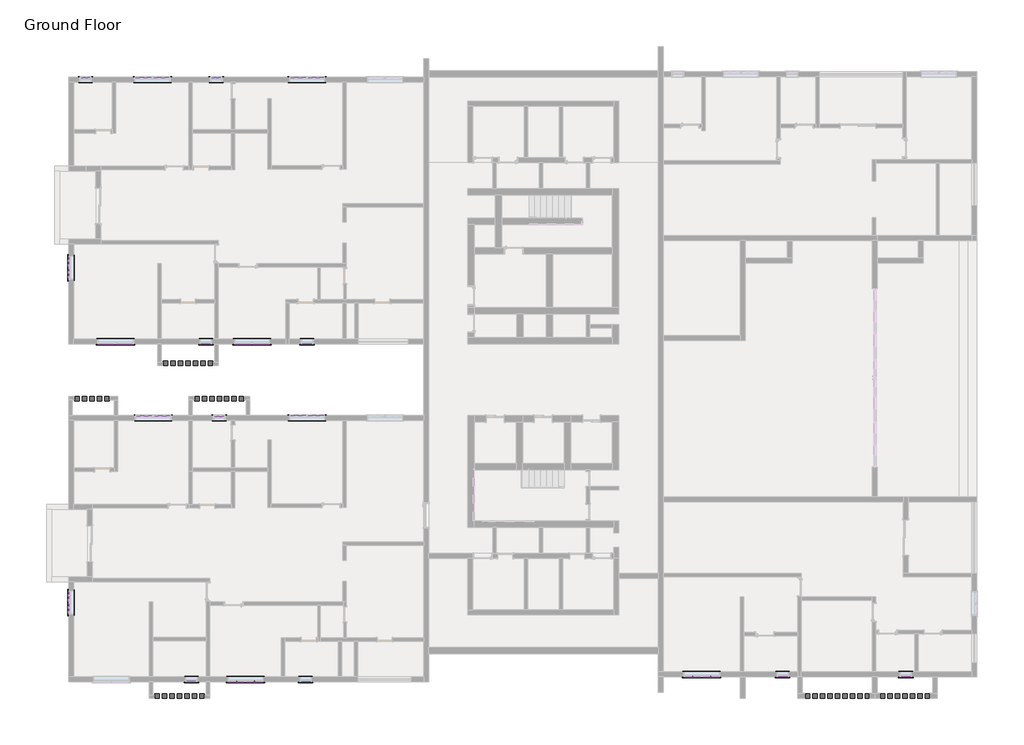
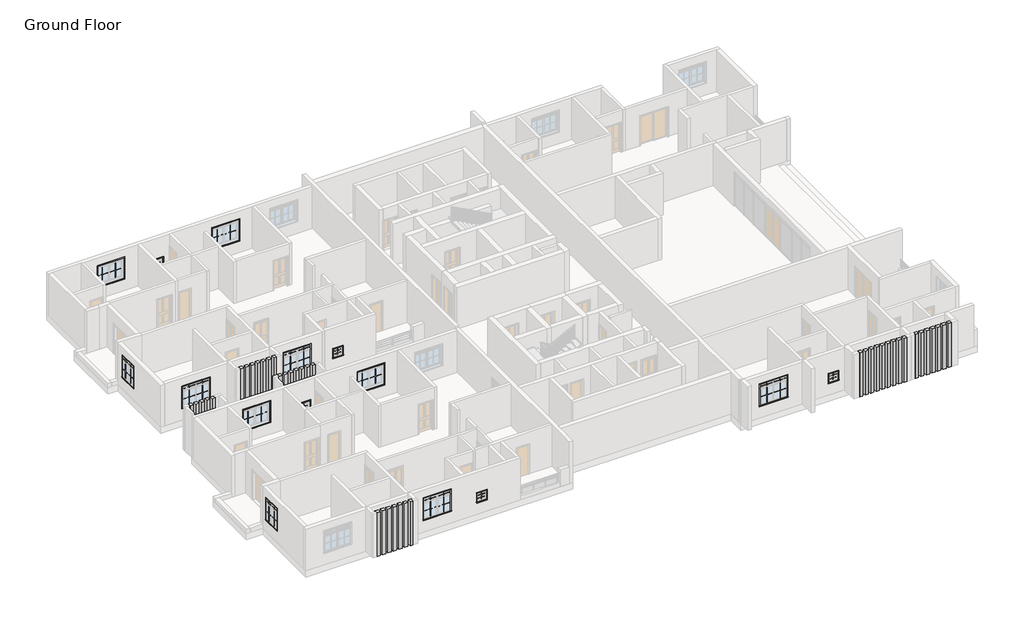
# One storey, part 8 of 9: 102 proxies.
"""IFC4 building model written with IfcOpenShell, lengths in millimetres."""

from ifc_helpers import new_model, si_unit, origin, place, context, project, spatial, transform, mapped, element, save
from components import generic_models_1_generic_models_1_04f99ef1, generic_models_2_generic_models_1_d649346d, generic_models_3_generic_models_1_029f251b, generic_models_4_generic_models_1_81c75abe, generic_models_5_generic_models_1_cca4fb08, generic_models_6_generic_models_1_46a45353, muntin_pattern_2x2_muntin_pattern_2x2_dc2504c2, muntin_pattern_2x2_muntin_pattern_2x2_0aa094e9, muntin_pattern_2x2_muntin_pattern_2x2_f17ebf58, muntin_pattern_2x2_muntin_pattern_2x2_cfeb24ad, muntin_pattern_2x2_muntin_pattern_2x2_4dfeb3f3, muntin_pattern_2x2_muntin_pattern_2x2_e852a7e4, muntin_pattern_2x2_muntin_pattern_2x2_3df65231, trim_window_exterior_flat_with_sill_c22f0c79, trim_window_exterior_flat_with_sill_858dc10d, trim_window_exterior_flat_with_sill_92b9b949, trim_window_interior_flat_picture_frame_d1f4d6ef, trim_window_interior_flat_picture_frame_3927330c, trim_window_interior_flat_picture_frame_3bb882cf

model = new_model("IFC4")

# Units and contexts
model_context = context("Model", 3, world=origin())
ifc_project = project(units=[si_unit("LENGTHUNIT", "METRE", prefix="MILLI")], contexts=[model_context])

# Site, building, storey
site = spatial("IfcSite", under=ifc_project)
building = spatial("IfcBuilding", under=site)
storey = spatial("IfcBuildingStorey", under=building, Name="Ground Floor", Elevation=0.0)

# Proxies
placement = place(None, origin())
generic_models_1_generic_models_1_shape = generic_models_1_generic_models_1_04f99ef1(model_context)
element("IfcBuildingElementProxy", 1, Name="Generic Models 1 : Generic Models 1", ObjectType="Generic Models 1 : Generic Models 1", at=placement, inside=storey, context=model_context, shape_type="MappedRepresentation", body=[
    mapped(generic_models_1_generic_models_1_shape, transform((0.0, 0.0, 0.0), x_axis=(1.0, 0.0, 0.0), y_axis=(0.0, 1.0, 0.0), z_axis=(0.0, 0.0, 1.0))),
])
generic_models_2_generic_models_1_shape = generic_models_2_generic_models_1_d649346d(model_context)
element("IfcBuildingElementProxy", 2, Name="Generic Models 2 : Generic Models 1", ObjectType="Generic Models 2 : Generic Models 1", at=placement, inside=storey, context=model_context, shape_type="MappedRepresentation", body=[
    mapped(generic_models_2_generic_models_1_shape, transform((0.0, 0.0, 0.0), x_axis=(1.0, 0.0, 0.0), y_axis=(0.0, 1.0, 0.0), z_axis=(0.0, 0.0, 1.0))),
])
generic_models_3_generic_models_1_shape = generic_models_3_generic_models_1_029f251b(model_context)
element("IfcBuildingElementProxy", 3, Name="Generic Models 3 : Generic Models 1", ObjectType="Generic Models 3 : Generic Models 1", at=placement, inside=storey, context=model_context, shape_type="MappedRepresentation", body=[
    mapped(generic_models_3_generic_models_1_shape, transform((-38.1, 0.0, 0.0), x_axis=(1.0, 0.0, 0.0), y_axis=(0.0, 1.0, 0.0), z_axis=(0.0, 0.0, 1.0))),
])
generic_models_4_generic_models_1_shape = generic_models_4_generic_models_1_81c75abe(model_context)
element("IfcBuildingElementProxy", 4, Name="Generic Models 4 : Generic Models 1", ObjectType="Generic Models 4 : Generic Models 1", at=placement, inside=storey, context=model_context, shape_type="MappedRepresentation", body=[
    mapped(generic_models_4_generic_models_1_shape, transform((-38.1, 0.0, 0.0), x_axis=(1.0, 0.0, 0.0), y_axis=(0.0, 1.0, 0.0), z_axis=(0.0, 0.0, 1.0))),
])
generic_models_5_generic_models_1_shape = generic_models_5_generic_models_1_cca4fb08(model_context)
element("IfcBuildingElementProxy", 5, Name="Generic Models 5 : Generic Models 1", ObjectType="Generic Models 5 : Generic Models 1", at=placement, inside=storey, context=model_context, shape_type="MappedRepresentation", body=[
    mapped(generic_models_5_generic_models_1_shape, transform((25.4, 0.0, 0.0), x_axis=(1.0, 0.0, 0.0), y_axis=(0.0, 1.0, 0.0), z_axis=(0.0, 0.0, 1.0))),
])
generic_models_6_generic_models_1_shape = generic_models_6_generic_models_1_46a45353(model_context)
element("IfcBuildingElementProxy", 6, Name="Generic Models 6 : Generic Models 1", ObjectType="Generic Models 6 : Generic Models 1", at=placement, inside=storey, context=model_context, shape_type="MappedRepresentation", body=[
    mapped(generic_models_6_generic_models_1_shape, transform((-38.1, 0.0, 0.0), x_axis=(1.0, 0.0, 0.0), y_axis=(0.0, 1.0, 0.0), z_axis=(0.0, 0.0, 1.0))),
])
muntin_pattern_2x2_muntin_pattern_2x2_shape = muntin_pattern_2x2_muntin_pattern_2x2_dc2504c2(model_context)
element("IfcBuildingElementProxy", 7, Name="Muntin Pattern_2x2 : Muntin Pattern_2x2", ObjectType="Muntin Pattern_2x2 : Muntin Pattern_2x2", at=placement, inside=storey, context=model_context, shape_type="MappedRepresentation", body=[
    mapped(muntin_pattern_2x2_muntin_pattern_2x2_shape, transform((-4881.5328682, -1988.440108, 984.25), x_axis=(-1.0, 0.0, 0.0), y_axis=(0.0, -1.0, 0.0), z_axis=(0.0, 0.0, 1.0))),
])
element("IfcBuildingElementProxy", 8, Name="Muntin Pattern_2x2 : Muntin Pattern_2x2", ObjectType="Muntin Pattern_2x2 : Muntin Pattern_2x2", at=placement, inside=storey, context=model_context, shape_type="MappedRepresentation", body=[
    mapped(muntin_pattern_2x2_muntin_pattern_2x2_shape, transform((-10517.1578682, 11632.309892, 984.25), x_axis=(1.0, 0.0, 0.0), y_axis=(0.0, 1.0, 0.0), z_axis=(0.0, 0.0, 1.0))),
])
element("IfcBuildingElementProxy", 9, Name="Muntin Pattern_2x2 : Muntin Pattern_2x2", ObjectType="Muntin Pattern_2x2 : Muntin Pattern_2x2", at=placement, inside=storey, context=model_context, shape_type="MappedRepresentation", body=[
    mapped(muntin_pattern_2x2_muntin_pattern_2x2_shape, transform((-2643.1578682, 11632.309892, 984.25), x_axis=(1.0, 0.0, 0.0), y_axis=(0.0, 1.0, 0.0), z_axis=(0.0, 0.0, 1.0))),
])
element("IfcBuildingElementProxy", 10, Name="Muntin Pattern_2x2 : Muntin Pattern_2x2", ObjectType="Muntin Pattern_2x2 : Muntin Pattern_2x2", at=placement, inside=storey, context=model_context, shape_type="MappedRepresentation", body=[
    mapped(muntin_pattern_2x2_muntin_pattern_2x2_shape, transform((-11529.9828682, 15308.959892, 984.25), x_axis=(-1.0, 0.0, 0.0), y_axis=(0.0, -1.0, 0.0), z_axis=(0.0, 0.0, 1.0))),
])
element("IfcBuildingElementProxy", 11, Name="Muntin Pattern_2x2 : Muntin Pattern_2x2", ObjectType="Muntin Pattern_2x2 : Muntin Pattern_2x2", at=placement, inside=storey, context=model_context, shape_type="MappedRepresentation", body=[
    mapped(muntin_pattern_2x2_muntin_pattern_2x2_shape, transform((-4551.3328682, 15308.959892, 984.25), x_axis=(-1.0, 0.0, 0.0), y_axis=(0.0, -1.0, 0.0), z_axis=(0.0, 0.0, 1.0))),
])
element("IfcBuildingElementProxy", 12, Name="Muntin Pattern_2x2 : Muntin Pattern_2x2", ObjectType="Muntin Pattern_2x2 : Muntin Pattern_2x2", at=placement, inside=storey, context=model_context, shape_type="MappedRepresentation", body=[
    mapped(muntin_pattern_2x2_muntin_pattern_2x2_shape, transform((-10561.6078682, 28955.109892, 984.25), x_axis=(1.0, 0.0, 0.0), y_axis=(0.0, 1.0, 0.0), z_axis=(0.0, 0.0, 1.0))),
])
element("IfcBuildingElementProxy", 13, Name="Muntin Pattern_2x2 : Muntin Pattern_2x2", ObjectType="Muntin Pattern_2x2 : Muntin Pattern_2x2", at=placement, inside=storey, context=model_context, shape_type="MappedRepresentation", body=[
    mapped(muntin_pattern_2x2_muntin_pattern_2x2_shape, transform((-2643.1578682, 28955.109892, 984.25), x_axis=(1.0, 0.0, 0.0), y_axis=(0.0, 1.0, 0.0), z_axis=(0.0, 0.0, 1.0))),
])
element("IfcBuildingElementProxy", 14, Name="Muntin Pattern_2x2 : Muntin Pattern_2x2", ObjectType="Muntin Pattern_2x2 : Muntin Pattern_2x2", at=placement, inside=storey, context=model_context, shape_type="MappedRepresentation", body=[
    mapped(muntin_pattern_2x2_muntin_pattern_2x2_shape, transform((18461.0671318, -1734.440108, 984.25), x_axis=(-1.0, 0.0, 0.0), y_axis=(0.0, -1.0, 0.0), z_axis=(0.0, 0.0, 1.0))),
])
muntin_pattern_2x2_muntin_pattern_2x2_2_shape = muntin_pattern_2x2_muntin_pattern_2x2_0aa094e9(model_context)
element("IfcBuildingElementProxy", 15, Name="Muntin Pattern_2x2 : Muntin Pattern_2x2", ObjectType="Muntin Pattern_2x2 : Muntin Pattern_2x2", at=placement, inside=storey, context=model_context, shape_type="MappedRepresentation", body=[
    mapped(muntin_pattern_2x2_muntin_pattern_2x2_2_shape, transform((-5792.7578682, -1988.440108, 984.25), x_axis=(1.0, 0.0, 0.0), y_axis=(0.0, 1.0, 0.0), z_axis=(0.0, 0.0, 1.0))),
])
element("IfcBuildingElementProxy", 16, Name="Muntin Pattern_2x2 : Muntin Pattern_2x2", ObjectType="Muntin Pattern_2x2 : Muntin Pattern_2x2", at=placement, inside=storey, context=model_context, shape_type="MappedRepresentation", body=[
    mapped(muntin_pattern_2x2_muntin_pattern_2x2_2_shape, transform((-9605.9328682, 11632.309892, 984.25), x_axis=(-1.0, 0.0, 0.0), y_axis=(0.0, -1.0, 0.0), z_axis=(0.0, 0.0, 1.0))),
])
element("IfcBuildingElementProxy", 17, Name="Muntin Pattern_2x2 : Muntin Pattern_2x2", ObjectType="Muntin Pattern_2x2 : Muntin Pattern_2x2", at=placement, inside=storey, context=model_context, shape_type="MappedRepresentation", body=[
    mapped(muntin_pattern_2x2_muntin_pattern_2x2_2_shape, transform((-1731.9328682, 11632.309892, 984.25), x_axis=(-1.0, 0.0, 0.0), y_axis=(0.0, -1.0, 0.0), z_axis=(0.0, 0.0, 1.0))),
])
element("IfcBuildingElementProxy", 18, Name="Muntin Pattern_2x2 : Muntin Pattern_2x2", ObjectType="Muntin Pattern_2x2 : Muntin Pattern_2x2", at=placement, inside=storey, context=model_context, shape_type="MappedRepresentation", body=[
    mapped(muntin_pattern_2x2_muntin_pattern_2x2_2_shape, transform((-12441.2078682, 15308.959892, 984.25), x_axis=(1.0, 0.0, 0.0), y_axis=(0.0, 1.0, 0.0), z_axis=(0.0, 0.0, 1.0))),
])
element("IfcBuildingElementProxy", 19, Name="Muntin Pattern_2x2 : Muntin Pattern_2x2", ObjectType="Muntin Pattern_2x2 : Muntin Pattern_2x2", at=placement, inside=storey, context=model_context, shape_type="MappedRepresentation", body=[
    mapped(muntin_pattern_2x2_muntin_pattern_2x2_2_shape, transform((-5462.5578682, 15308.959892, 984.25), x_axis=(1.0, 0.0, 0.0), y_axis=(0.0, 1.0, 0.0), z_axis=(0.0, 0.0, 1.0))),
])
element("IfcBuildingElementProxy", 20, Name="Muntin Pattern_2x2 : Muntin Pattern_2x2", ObjectType="Muntin Pattern_2x2 : Muntin Pattern_2x2", at=placement, inside=storey, context=model_context, shape_type="MappedRepresentation", body=[
    mapped(muntin_pattern_2x2_muntin_pattern_2x2_2_shape, transform((-9650.3828682, 28955.109892, 984.25), x_axis=(-1.0, 0.0, 0.0), y_axis=(0.0, -1.0, 0.0), z_axis=(0.0, 0.0, 1.0))),
])
element("IfcBuildingElementProxy", 21, Name="Muntin Pattern_2x2 : Muntin Pattern_2x2", ObjectType="Muntin Pattern_2x2 : Muntin Pattern_2x2", at=placement, inside=storey, context=model_context, shape_type="MappedRepresentation", body=[
    mapped(muntin_pattern_2x2_muntin_pattern_2x2_2_shape, transform((-1731.9328682, 28955.109892, 984.25), x_axis=(-1.0, 0.0, 0.0), y_axis=(0.0, -1.0, 0.0), z_axis=(0.0, 0.0, 1.0))),
])
element("IfcBuildingElementProxy", 22, Name="Muntin Pattern_2x2 : Muntin Pattern_2x2", ObjectType="Muntin Pattern_2x2 : Muntin Pattern_2x2", at=placement, inside=storey, context=model_context, shape_type="MappedRepresentation", body=[
    mapped(muntin_pattern_2x2_muntin_pattern_2x2_2_shape, transform((17549.8421318, -1734.440108, 984.25), x_axis=(1.0, 0.0, 0.0), y_axis=(0.0, 1.0, 0.0), z_axis=(0.0, 0.0, 1.0))),
])
muntin_pattern_2x2_muntin_pattern_2x2_3_shape = muntin_pattern_2x2_muntin_pattern_2x2_f17ebf58(model_context)
element("IfcBuildingElementProxy", 23, Name="Muntin Pattern_2x2 : Muntin Pattern_2x2", ObjectType="Muntin Pattern_2x2 : Muntin Pattern_2x2", at=placement, inside=storey, context=model_context, shape_type="MappedRepresentation", body=[
    mapped(muntin_pattern_2x2_muntin_pattern_2x2_3_shape, transform((-5792.7578682, -1988.440108, 2203.45), x_axis=(1.0, 0.0, 0.0), y_axis=(0.0, 1.0, 0.0), z_axis=(0.0, 0.0, 1.0))),
])
element("IfcBuildingElementProxy", 24, Name="Muntin Pattern_2x2 : Muntin Pattern_2x2", ObjectType="Muntin Pattern_2x2 : Muntin Pattern_2x2", at=placement, inside=storey, context=model_context, shape_type="MappedRepresentation", body=[
    mapped(muntin_pattern_2x2_muntin_pattern_2x2_3_shape, transform((-4881.5328682, -1988.440108, 2203.45), x_axis=(1.0, 0.0, 0.0), y_axis=(0.0, 1.0, 0.0), z_axis=(0.0, 0.0, 1.0))),
])
element("IfcBuildingElementProxy", 25, Name="Muntin Pattern_2x2 : Muntin Pattern_2x2", ObjectType="Muntin Pattern_2x2 : Muntin Pattern_2x2", at=placement, inside=storey, context=model_context, shape_type="MappedRepresentation", body=[
    mapped(muntin_pattern_2x2_muntin_pattern_2x2_3_shape, transform((-9605.9328682, 11632.309892, 2203.45), x_axis=(-1.0, 0.0, 0.0), y_axis=(0.0, -1.0, 0.0), z_axis=(0.0, 0.0, 1.0))),
])
element("IfcBuildingElementProxy", 26, Name="Muntin Pattern_2x2 : Muntin Pattern_2x2", ObjectType="Muntin Pattern_2x2 : Muntin Pattern_2x2", at=placement, inside=storey, context=model_context, shape_type="MappedRepresentation", body=[
    mapped(muntin_pattern_2x2_muntin_pattern_2x2_3_shape, transform((-10517.1578682, 11632.309892, 2203.45), x_axis=(-1.0, 0.0, 0.0), y_axis=(0.0, -1.0, 0.0), z_axis=(0.0, 0.0, 1.0))),
])
element("IfcBuildingElementProxy", 27, Name="Muntin Pattern_2x2 : Muntin Pattern_2x2", ObjectType="Muntin Pattern_2x2 : Muntin Pattern_2x2", at=placement, inside=storey, context=model_context, shape_type="MappedRepresentation", body=[
    mapped(muntin_pattern_2x2_muntin_pattern_2x2_3_shape, transform((-1731.9328682, 11632.309892, 2203.45), x_axis=(-1.0, 0.0, 0.0), y_axis=(0.0, -1.0, 0.0), z_axis=(0.0, 0.0, 1.0))),
])
element("IfcBuildingElementProxy", 28, Name="Muntin Pattern_2x2 : Muntin Pattern_2x2", ObjectType="Muntin Pattern_2x2 : Muntin Pattern_2x2", at=placement, inside=storey, context=model_context, shape_type="MappedRepresentation", body=[
    mapped(muntin_pattern_2x2_muntin_pattern_2x2_3_shape, transform((-2643.1578682, 11632.309892, 2203.45), x_axis=(-1.0, 0.0, 0.0), y_axis=(0.0, -1.0, 0.0), z_axis=(0.0, 0.0, 1.0))),
])
element("IfcBuildingElementProxy", 29, Name="Muntin Pattern_2x2 : Muntin Pattern_2x2", ObjectType="Muntin Pattern_2x2 : Muntin Pattern_2x2", at=placement, inside=storey, context=model_context, shape_type="MappedRepresentation", body=[
    mapped(muntin_pattern_2x2_muntin_pattern_2x2_3_shape, transform((-12441.2078682, 15308.959892, 2203.45), x_axis=(1.0, 0.0, 0.0), y_axis=(0.0, 1.0, 0.0), z_axis=(0.0, 0.0, 1.0))),
])
element("IfcBuildingElementProxy", 30, Name="Muntin Pattern_2x2 : Muntin Pattern_2x2", ObjectType="Muntin Pattern_2x2 : Muntin Pattern_2x2", at=placement, inside=storey, context=model_context, shape_type="MappedRepresentation", body=[
    mapped(muntin_pattern_2x2_muntin_pattern_2x2_3_shape, transform((-11529.9828682, 15308.959892, 2203.45), x_axis=(1.0, 0.0, 0.0), y_axis=(0.0, 1.0, 0.0), z_axis=(0.0, 0.0, 1.0))),
])
element("IfcBuildingElementProxy", 31, Name="Muntin Pattern_2x2 : Muntin Pattern_2x2", ObjectType="Muntin Pattern_2x2 : Muntin Pattern_2x2", at=placement, inside=storey, context=model_context, shape_type="MappedRepresentation", body=[
    mapped(muntin_pattern_2x2_muntin_pattern_2x2_3_shape, transform((-5462.5578682, 15308.959892, 2203.45), x_axis=(1.0, 0.0, 0.0), y_axis=(0.0, 1.0, 0.0), z_axis=(0.0, 0.0, 1.0))),
])
element("IfcBuildingElementProxy", 32, Name="Muntin Pattern_2x2 : Muntin Pattern_2x2", ObjectType="Muntin Pattern_2x2 : Muntin Pattern_2x2", at=placement, inside=storey, context=model_context, shape_type="MappedRepresentation", body=[
    mapped(muntin_pattern_2x2_muntin_pattern_2x2_3_shape, transform((-4551.3328682, 15308.959892, 2203.45), x_axis=(1.0, 0.0, 0.0), y_axis=(0.0, 1.0, 0.0), z_axis=(0.0, 0.0, 1.0))),
])
element("IfcBuildingElementProxy", 33, Name="Muntin Pattern_2x2 : Muntin Pattern_2x2", ObjectType="Muntin Pattern_2x2 : Muntin Pattern_2x2", at=placement, inside=storey, context=model_context, shape_type="MappedRepresentation", body=[
    mapped(muntin_pattern_2x2_muntin_pattern_2x2_3_shape, transform((-9650.3828682, 28955.109892, 2203.45), x_axis=(-1.0, 0.0, 0.0), y_axis=(0.0, -1.0, 0.0), z_axis=(0.0, 0.0, 1.0))),
])
element("IfcBuildingElementProxy", 34, Name="Muntin Pattern_2x2 : Muntin Pattern_2x2", ObjectType="Muntin Pattern_2x2 : Muntin Pattern_2x2", at=placement, inside=storey, context=model_context, shape_type="MappedRepresentation", body=[
    mapped(muntin_pattern_2x2_muntin_pattern_2x2_3_shape, transform((-10561.6078682, 28955.109892, 2203.45), x_axis=(-1.0, 0.0, 0.0), y_axis=(0.0, -1.0, 0.0), z_axis=(0.0, 0.0, 1.0))),
])
element("IfcBuildingElementProxy", 35, Name="Muntin Pattern_2x2 : Muntin Pattern_2x2", ObjectType="Muntin Pattern_2x2 : Muntin Pattern_2x2", at=placement, inside=storey, context=model_context, shape_type="MappedRepresentation", body=[
    mapped(muntin_pattern_2x2_muntin_pattern_2x2_3_shape, transform((-1731.9328682, 28955.109892, 2203.45), x_axis=(-1.0, 0.0, 0.0), y_axis=(0.0, -1.0, 0.0), z_axis=(0.0, 0.0, 1.0))),
])
element("IfcBuildingElementProxy", 36, Name="Muntin Pattern_2x2 : Muntin Pattern_2x2", ObjectType="Muntin Pattern_2x2 : Muntin Pattern_2x2", at=placement, inside=storey, context=model_context, shape_type="MappedRepresentation", body=[
    mapped(muntin_pattern_2x2_muntin_pattern_2x2_3_shape, transform((-2643.1578682, 28955.109892, 2203.45), x_axis=(-1.0, 0.0, 0.0), y_axis=(0.0, -1.0, 0.0), z_axis=(0.0, 0.0, 1.0))),
])
element("IfcBuildingElementProxy", 37, Name="Muntin Pattern_2x2 : Muntin Pattern_2x2", ObjectType="Muntin Pattern_2x2 : Muntin Pattern_2x2", at=placement, inside=storey, context=model_context, shape_type="MappedRepresentation", body=[
    mapped(muntin_pattern_2x2_muntin_pattern_2x2_3_shape, transform((17549.8421318, -1734.440108, 2203.45), x_axis=(1.0, 0.0, 0.0), y_axis=(0.0, 1.0, 0.0), z_axis=(0.0, 0.0, 1.0))),
])
element("IfcBuildingElementProxy", 38, Name="Muntin Pattern_2x2 : Muntin Pattern_2x2", ObjectType="Muntin Pattern_2x2 : Muntin Pattern_2x2", at=placement, inside=storey, context=model_context, shape_type="MappedRepresentation", body=[
    mapped(muntin_pattern_2x2_muntin_pattern_2x2_3_shape, transform((18461.0671318, -1734.440108, 2203.45), x_axis=(1.0, 0.0, 0.0), y_axis=(0.0, 1.0, 0.0), z_axis=(0.0, 0.0, 1.0))),
])
muntin_pattern_2x2_muntin_pattern_2x2_4_shape = muntin_pattern_2x2_muntin_pattern_2x2_cfeb24ad(model_context)
element("IfcBuildingElementProxy", 39, Name="Muntin Pattern_2x2 : Muntin Pattern_2x2", ObjectType="Muntin Pattern_2x2 : Muntin Pattern_2x2", at=placement, inside=storey, context=model_context, shape_type="MappedRepresentation", body=[
    mapped(muntin_pattern_2x2_muntin_pattern_2x2_4_shape, transform((-13528.6453682, 28929.709892, 1241.425), x_axis=(1.0, 0.0, 0.0), y_axis=(0.0, 1.0, 0.0), z_axis=(0.0, 0.0, 1.0))),
])
element("IfcBuildingElementProxy", 40, Name="Muntin Pattern_2x2 : Muntin Pattern_2x2", ObjectType="Muntin Pattern_2x2 : Muntin Pattern_2x2", at=placement, inside=storey, context=model_context, shape_type="MappedRepresentation", body=[
    mapped(muntin_pattern_2x2_muntin_pattern_2x2_4_shape, transform((-13528.6453682, 28885.259892, 990.6), x_axis=(1.0, 0.0, 0.0), y_axis=(0.0, 1.0, 0.0), z_axis=(0.0, 0.0, 1.0))),
])
element("IfcBuildingElementProxy", 41, Name="Muntin Pattern_2x2 : Muntin Pattern_2x2", ObjectType="Muntin Pattern_2x2 : Muntin Pattern_2x2", at=placement, inside=storey, context=model_context, shape_type="MappedRepresentation", body=[
    mapped(muntin_pattern_2x2_muntin_pattern_2x2_4_shape, transform((-6835.7453682, 28929.709892, 1241.425), x_axis=(1.0, 0.0, 0.0), y_axis=(0.0, 1.0, 0.0), z_axis=(0.0, 0.0, 1.0))),
])
element("IfcBuildingElementProxy", 42, Name="Muntin Pattern_2x2 : Muntin Pattern_2x2", ObjectType="Muntin Pattern_2x2 : Muntin Pattern_2x2", at=placement, inside=storey, context=model_context, shape_type="MappedRepresentation", body=[
    mapped(muntin_pattern_2x2_muntin_pattern_2x2_4_shape, transform((-6835.7453682, 28885.259892, 990.6), x_axis=(1.0, 0.0, 0.0), y_axis=(0.0, 1.0, 0.0), z_axis=(0.0, 0.0, 1.0))),
])
element("IfcBuildingElementProxy", 43, Name="Muntin Pattern_2x2 : Muntin Pattern_2x2", ObjectType="Muntin Pattern_2x2 : Muntin Pattern_2x2", at=placement, inside=storey, context=model_context, shape_type="MappedRepresentation", body=[
    mapped(muntin_pattern_2x2_muntin_pattern_2x2_4_shape, transform((-7369.1453682, 15334.359892, 1241.425), x_axis=(-1.0, 0.0, 0.0), y_axis=(0.0, -1.0, 0.0), z_axis=(0.0, 0.0, 1.0))),
])
element("IfcBuildingElementProxy", 44, Name="Muntin Pattern_2x2 : Muntin Pattern_2x2", ObjectType="Muntin Pattern_2x2 : Muntin Pattern_2x2", at=placement, inside=storey, context=model_context, shape_type="MappedRepresentation", body=[
    mapped(muntin_pattern_2x2_muntin_pattern_2x2_4_shape, transform((-7369.1453682, 15378.809892, 990.6), x_axis=(-1.0, 0.0, 0.0), y_axis=(0.0, -1.0, 0.0), z_axis=(0.0, 0.0, 1.0))),
])
element("IfcBuildingElementProxy", 45, Name="Muntin Pattern_2x2 : Muntin Pattern_2x2", ObjectType="Muntin Pattern_2x2 : Muntin Pattern_2x2", at=placement, inside=storey, context=model_context, shape_type="MappedRepresentation", body=[
    mapped(muntin_pattern_2x2_muntin_pattern_2x2_4_shape, transform((-2187.5453682, 15334.359892, 1241.425), x_axis=(-1.0, 0.0, 0.0), y_axis=(0.0, -1.0, 0.0), z_axis=(0.0, 0.0, 1.0))),
])
element("IfcBuildingElementProxy", 46, Name="Muntin Pattern_2x2 : Muntin Pattern_2x2", ObjectType="Muntin Pattern_2x2 : Muntin Pattern_2x2", at=placement, inside=storey, context=model_context, shape_type="MappedRepresentation", body=[
    mapped(muntin_pattern_2x2_muntin_pattern_2x2_4_shape, transform((-2187.5453682, 15378.809892, 990.6), x_axis=(-1.0, 0.0, 0.0), y_axis=(0.0, -1.0, 0.0), z_axis=(0.0, 0.0, 1.0))),
])
element("IfcBuildingElementProxy", 47, Name="Muntin Pattern_2x2 : Muntin Pattern_2x2", ObjectType="Muntin Pattern_2x2 : Muntin Pattern_2x2", at=placement, inside=storey, context=model_context, shape_type="MappedRepresentation", body=[
    mapped(muntin_pattern_2x2_muntin_pattern_2x2_4_shape, transform((-6683.3453682, 11606.909892, 1241.425), x_axis=(1.0, 0.0, 0.0), y_axis=(0.0, 1.0, 0.0), z_axis=(0.0, 0.0, 1.0))),
])
element("IfcBuildingElementProxy", 48, Name="Muntin Pattern_2x2 : Muntin Pattern_2x2", ObjectType="Muntin Pattern_2x2 : Muntin Pattern_2x2", at=placement, inside=storey, context=model_context, shape_type="MappedRepresentation", body=[
    mapped(muntin_pattern_2x2_muntin_pattern_2x2_4_shape, transform((-6683.3453682, 11562.459892, 990.6), x_axis=(1.0, 0.0, 0.0), y_axis=(0.0, 1.0, 0.0), z_axis=(0.0, 0.0, 1.0))),
])
element("IfcBuildingElementProxy", 49, Name="Muntin Pattern_2x2 : Muntin Pattern_2x2", ObjectType="Muntin Pattern_2x2 : Muntin Pattern_2x2", at=placement, inside=storey, context=model_context, shape_type="MappedRepresentation", body=[
    mapped(muntin_pattern_2x2_muntin_pattern_2x2_4_shape, transform((-8105.7453682, -1963.040108, 1241.425), x_axis=(-1.0, 0.0, 0.0), y_axis=(0.0, -1.0, 0.0), z_axis=(0.0, 0.0, 1.0))),
])
element("IfcBuildingElementProxy", 50, Name="Muntin Pattern_2x2 : Muntin Pattern_2x2", ObjectType="Muntin Pattern_2x2 : Muntin Pattern_2x2", at=placement, inside=storey, context=model_context, shape_type="MappedRepresentation", body=[
    mapped(muntin_pattern_2x2_muntin_pattern_2x2_4_shape, transform((-8105.7453682, -1918.590108, 990.6), x_axis=(-1.0, 0.0, 0.0), y_axis=(0.0, -1.0, 0.0), z_axis=(0.0, 0.0, 1.0))),
])
element("IfcBuildingElementProxy", 51, Name="Muntin Pattern_2x2 : Muntin Pattern_2x2", ObjectType="Muntin Pattern_2x2 : Muntin Pattern_2x2", at=placement, inside=storey, context=model_context, shape_type="MappedRepresentation", body=[
    mapped(muntin_pattern_2x2_muntin_pattern_2x2_4_shape, transform((-2263.7453682, -1963.040108, 1241.425), x_axis=(-1.0, 0.0, 0.0), y_axis=(0.0, -1.0, 0.0), z_axis=(0.0, 0.0, 1.0))),
])
element("IfcBuildingElementProxy", 52, Name="Muntin Pattern_2x2 : Muntin Pattern_2x2", ObjectType="Muntin Pattern_2x2 : Muntin Pattern_2x2", at=placement, inside=storey, context=model_context, shape_type="MappedRepresentation", body=[
    mapped(muntin_pattern_2x2_muntin_pattern_2x2_4_shape, transform((-2263.7453682, -1918.590108, 990.6), x_axis=(-1.0, 0.0, 0.0), y_axis=(0.0, -1.0, 0.0), z_axis=(0.0, 0.0, 1.0))),
])
element("IfcBuildingElementProxy", 53, Name="Muntin Pattern_2x2 : Muntin Pattern_2x2", ObjectType="Muntin Pattern_2x2 : Muntin Pattern_2x2", at=placement, inside=storey, context=model_context, shape_type="MappedRepresentation", body=[
    mapped(muntin_pattern_2x2_muntin_pattern_2x2_4_shape, transform((22145.6546318, -1709.040108, 1241.425), x_axis=(-1.0, 0.0, 0.0), y_axis=(0.0, -1.0, 0.0), z_axis=(0.0, 0.0, 1.0))),
])
element("IfcBuildingElementProxy", 54, Name="Muntin Pattern_2x2 : Muntin Pattern_2x2", ObjectType="Muntin Pattern_2x2 : Muntin Pattern_2x2", at=placement, inside=storey, context=model_context, shape_type="MappedRepresentation", body=[
    mapped(muntin_pattern_2x2_muntin_pattern_2x2_4_shape, transform((22145.6546318, -1664.590108, 990.6), x_axis=(-1.0, 0.0, 0.0), y_axis=(0.0, -1.0, 0.0), z_axis=(0.0, 0.0, 1.0))),
])
element("IfcBuildingElementProxy", 55, Name="Muntin Pattern_2x2 : Muntin Pattern_2x2", ObjectType="Muntin Pattern_2x2 : Muntin Pattern_2x2", at=placement, inside=storey, context=model_context, shape_type="MappedRepresentation", body=[
    mapped(muntin_pattern_2x2_muntin_pattern_2x2_4_shape, transform((28444.8546318, -1709.040108, 1241.425), x_axis=(-1.0, 0.0, 0.0), y_axis=(0.0, -1.0, 0.0), z_axis=(0.0, 0.0, 1.0))),
])
element("IfcBuildingElementProxy", 56, Name="Muntin Pattern_2x2 : Muntin Pattern_2x2", ObjectType="Muntin Pattern_2x2 : Muntin Pattern_2x2", at=placement, inside=storey, context=model_context, shape_type="MappedRepresentation", body=[
    mapped(muntin_pattern_2x2_muntin_pattern_2x2_4_shape, transform((28444.8546318, -1664.590108, 990.6), x_axis=(-1.0, 0.0, 0.0), y_axis=(0.0, -1.0, 0.0), z_axis=(0.0, 0.0, 1.0))),
])
muntin_pattern_2x2_muntin_pattern_2x2_5_shape = muntin_pattern_2x2_muntin_pattern_2x2_4dfeb3f3(model_context)
element("IfcBuildingElementProxy", 57, Name="Muntin Pattern_2x2 : Muntin Pattern_2x2", ObjectType="Muntin Pattern_2x2 : Muntin Pattern_2x2", at=placement, inside=storey, context=model_context, shape_type="MappedRepresentation", body=[
    mapped(muntin_pattern_2x2_muntin_pattern_2x2_5_shape, transform((-14382.7203682, 1762.822392, 984.25), x_axis=(0.0, 1.0, 0.0), y_axis=(-1.0, 0.0, 0.0), z_axis=(0.0, 0.0, 1.0))),
])
element("IfcBuildingElementProxy", 58, Name="Muntin Pattern_2x2 : Muntin Pattern_2x2", ObjectType="Muntin Pattern_2x2 : Muntin Pattern_2x2", at=placement, inside=storey, context=model_context, shape_type="MappedRepresentation", body=[
    mapped(muntin_pattern_2x2_muntin_pattern_2x2_5_shape, transform((-14382.7203682, 18907.822392, 984.25), x_axis=(0.0, 1.0, 0.0), y_axis=(-1.0, 0.0, 0.0), z_axis=(0.0, 0.0, 1.0))),
])
muntin_pattern_2x2_muntin_pattern_2x2_6_shape = muntin_pattern_2x2_muntin_pattern_2x2_e852a7e4(model_context)
element("IfcBuildingElementProxy", 59, Name="Muntin Pattern_2x2 : Muntin Pattern_2x2", ObjectType="Muntin Pattern_2x2 : Muntin Pattern_2x2", at=placement, inside=storey, context=model_context, shape_type="MappedRepresentation", body=[
    mapped(muntin_pattern_2x2_muntin_pattern_2x2_6_shape, transform((-14382.7203682, 2369.247392, 984.25), x_axis=(0.0, -1.0, 0.0), y_axis=(1.0, 0.0, 0.0), z_axis=(0.0, 0.0, 1.0))),
])
element("IfcBuildingElementProxy", 60, Name="Muntin Pattern_2x2 : Muntin Pattern_2x2", ObjectType="Muntin Pattern_2x2 : Muntin Pattern_2x2", at=placement, inside=storey, context=model_context, shape_type="MappedRepresentation", body=[
    mapped(muntin_pattern_2x2_muntin_pattern_2x2_6_shape, transform((-14382.7203682, 19514.247392, 984.25), x_axis=(0.0, -1.0, 0.0), y_axis=(1.0, 0.0, 0.0), z_axis=(0.0, 0.0, 1.0))),
])
muntin_pattern_2x2_muntin_pattern_2x2_7_shape = muntin_pattern_2x2_muntin_pattern_2x2_3df65231(model_context)
element("IfcBuildingElementProxy", 61, Name="Muntin Pattern_2x2 : Muntin Pattern_2x2", ObjectType="Muntin Pattern_2x2 : Muntin Pattern_2x2", at=placement, inside=storey, context=model_context, shape_type="MappedRepresentation", body=[
    mapped(muntin_pattern_2x2_muntin_pattern_2x2_7_shape, transform((-14382.7203682, 2369.247392, 2203.45), x_axis=(0.0, -1.0, 0.0), y_axis=(1.0, 0.0, 0.0), z_axis=(0.0, 0.0, 1.0))),
])
element("IfcBuildingElementProxy", 62, Name="Muntin Pattern_2x2 : Muntin Pattern_2x2", ObjectType="Muntin Pattern_2x2 : Muntin Pattern_2x2", at=placement, inside=storey, context=model_context, shape_type="MappedRepresentation", body=[
    mapped(muntin_pattern_2x2_muntin_pattern_2x2_7_shape, transform((-14382.7203682, 1762.822392, 2203.45), x_axis=(0.0, -1.0, 0.0), y_axis=(1.0, 0.0, 0.0), z_axis=(0.0, 0.0, 1.0))),
])
element("IfcBuildingElementProxy", 63, Name="Muntin Pattern_2x2 : Muntin Pattern_2x2", ObjectType="Muntin Pattern_2x2 : Muntin Pattern_2x2", at=placement, inside=storey, context=model_context, shape_type="MappedRepresentation", body=[
    mapped(muntin_pattern_2x2_muntin_pattern_2x2_7_shape, transform((-14382.7203682, 19514.247392, 2203.45), x_axis=(0.0, -1.0, 0.0), y_axis=(1.0, 0.0, 0.0), z_axis=(0.0, 0.0, 1.0))),
])
element("IfcBuildingElementProxy", 64, Name="Muntin Pattern_2x2 : Muntin Pattern_2x2", ObjectType="Muntin Pattern_2x2 : Muntin Pattern_2x2", at=placement, inside=storey, context=model_context, shape_type="MappedRepresentation", body=[
    mapped(muntin_pattern_2x2_muntin_pattern_2x2_7_shape, transform((-14382.7203682, 18907.822392, 2203.45), x_axis=(0.0, -1.0, 0.0), y_axis=(1.0, 0.0, 0.0), z_axis=(0.0, 0.0, 1.0))),
])
trim_window_exterior_flat_with_sill_shape = trim_window_exterior_flat_with_sill_c22f0c79(model_context)
element("IfcBuildingElementProxy", 65, Name="Trim-Window-Exterior-Flat : with Sill", ObjectType="Trim-Window-Exterior-Flat : with Sill", at=placement, inside=storey, context=model_context, shape_type="MappedRepresentation", body=[
    mapped(trim_window_exterior_flat_with_sill_shape, transform((-5337.1453682, -1997.965108, 2438.4), x_axis=(1.0, 0.0, 0.0), y_axis=(0.0, 0.0, 1.0), z_axis=(0.0, -1.0, 0.0))),
])
element("IfcBuildingElementProxy", 66, Name="Trim-Window-Exterior-Flat : with Sill", ObjectType="Trim-Window-Exterior-Flat : with Sill", at=placement, inside=storey, context=model_context, shape_type="MappedRepresentation", body=[
    mapped(trim_window_exterior_flat_with_sill_shape, transform((-10061.5453682, 11641.834892, 2438.4), x_axis=(-1.0, 0.0, 0.0), y_axis=(0.0, 0.0, 1.0), z_axis=(0.0, 1.0, 0.0))),
])
element("IfcBuildingElementProxy", 67, Name="Trim-Window-Exterior-Flat : with Sill", ObjectType="Trim-Window-Exterior-Flat : with Sill", at=placement, inside=storey, context=model_context, shape_type="MappedRepresentation", body=[
    mapped(trim_window_exterior_flat_with_sill_shape, transform((-2187.5453682, 11641.834892, 2438.4), x_axis=(-1.0, 0.0, 0.0), y_axis=(0.0, 0.0, 1.0), z_axis=(0.0, 1.0, 0.0))),
])
element("IfcBuildingElementProxy", 68, Name="Trim-Window-Exterior-Flat : with Sill", ObjectType="Trim-Window-Exterior-Flat : with Sill", at=placement, inside=storey, context=model_context, shape_type="MappedRepresentation", body=[
    mapped(trim_window_exterior_flat_with_sill_shape, transform((-11985.5953682, 15299.434892, 2438.4), x_axis=(1.0, 0.0, 0.0), y_axis=(0.0, 0.0, 1.0), z_axis=(0.0, -1.0, 0.0))),
])
element("IfcBuildingElementProxy", 69, Name="Trim-Window-Exterior-Flat : with Sill", ObjectType="Trim-Window-Exterior-Flat : with Sill", at=placement, inside=storey, context=model_context, shape_type="MappedRepresentation", body=[
    mapped(trim_window_exterior_flat_with_sill_shape, transform((-5006.9453682, 15299.434892, 2438.4), x_axis=(1.0, 0.0, 0.0), y_axis=(0.0, 0.0, 1.0), z_axis=(0.0, -1.0, 0.0))),
])
element("IfcBuildingElementProxy", 70, Name="Trim-Window-Exterior-Flat : with Sill", ObjectType="Trim-Window-Exterior-Flat : with Sill", at=placement, inside=storey, context=model_context, shape_type="MappedRepresentation", body=[
    mapped(trim_window_exterior_flat_with_sill_shape, transform((-10105.9953682, 28964.634892, 2438.4), x_axis=(-1.0, 0.0, 0.0), y_axis=(0.0, 0.0, 1.0), z_axis=(0.0, 1.0, 0.0))),
])
element("IfcBuildingElementProxy", 71, Name="Trim-Window-Exterior-Flat : with Sill", ObjectType="Trim-Window-Exterior-Flat : with Sill", at=placement, inside=storey, context=model_context, shape_type="MappedRepresentation", body=[
    mapped(trim_window_exterior_flat_with_sill_shape, transform((-2187.5453682, 28964.634892, 2438.4), x_axis=(-1.0, 0.0, 0.0), y_axis=(0.0, 0.0, 1.0), z_axis=(0.0, 1.0, 0.0))),
])
element("IfcBuildingElementProxy", 72, Name="Trim-Window-Exterior-Flat : with Sill", ObjectType="Trim-Window-Exterior-Flat : with Sill", at=placement, inside=storey, context=model_context, shape_type="MappedRepresentation", body=[
    mapped(trim_window_exterior_flat_with_sill_shape, transform((18005.4546318, -1743.965108, 2438.4), x_axis=(1.0, 0.0, 0.0), y_axis=(0.0, 0.0, 1.0), z_axis=(0.0, -1.0, 0.0))),
])
trim_window_exterior_flat_with_sill_2_shape = trim_window_exterior_flat_with_sill_858dc10d(model_context)
element("IfcBuildingElementProxy", 73, Name="Trim-Window-Exterior-Flat : with Sill", ObjectType="Trim-Window-Exterior-Flat : with Sill", at=placement, inside=storey, context=model_context, shape_type="MappedRepresentation", body=[
    mapped(trim_window_exterior_flat_with_sill_2_shape, transform((-13528.6453682, 28964.634892, 1524.0), x_axis=(-1.0, 0.0, 0.0), y_axis=(0.0, 0.0, 1.0), z_axis=(0.0, 1.0, 0.0))),
])
element("IfcBuildingElementProxy", 74, Name="Trim-Window-Exterior-Flat : with Sill", ObjectType="Trim-Window-Exterior-Flat : with Sill", at=placement, inside=storey, context=model_context, shape_type="MappedRepresentation", body=[
    mapped(trim_window_exterior_flat_with_sill_2_shape, transform((-6835.7453682, 28964.634892, 1524.0), x_axis=(-1.0, 0.0, 0.0), y_axis=(0.0, 0.0, 1.0), z_axis=(0.0, 1.0, 0.0))),
])
element("IfcBuildingElementProxy", 75, Name="Trim-Window-Exterior-Flat : with Sill", ObjectType="Trim-Window-Exterior-Flat : with Sill", at=placement, inside=storey, context=model_context, shape_type="MappedRepresentation", body=[
    mapped(trim_window_exterior_flat_with_sill_2_shape, transform((-7369.1453682, 15299.434892, 1524.0), x_axis=(1.0, 0.0, 0.0), y_axis=(0.0, 0.0, 1.0), z_axis=(0.0, -1.0, 0.0))),
])
element("IfcBuildingElementProxy", 76, Name="Trim-Window-Exterior-Flat : with Sill", ObjectType="Trim-Window-Exterior-Flat : with Sill", at=placement, inside=storey, context=model_context, shape_type="MappedRepresentation", body=[
    mapped(trim_window_exterior_flat_with_sill_2_shape, transform((-2187.5453682, 15299.434892, 1524.0), x_axis=(1.0, 0.0, 0.0), y_axis=(0.0, 0.0, 1.0), z_axis=(0.0, -1.0, 0.0))),
])
element("IfcBuildingElementProxy", 77, Name="Trim-Window-Exterior-Flat : with Sill", ObjectType="Trim-Window-Exterior-Flat : with Sill", at=placement, inside=storey, context=model_context, shape_type="MappedRepresentation", body=[
    mapped(trim_window_exterior_flat_with_sill_2_shape, transform((-6683.3453682, 11641.834892, 1524.0), x_axis=(-1.0, 0.0, 0.0), y_axis=(0.0, 0.0, 1.0), z_axis=(0.0, 1.0, 0.0))),
])
element("IfcBuildingElementProxy", 78, Name="Trim-Window-Exterior-Flat : with Sill", ObjectType="Trim-Window-Exterior-Flat : with Sill", at=placement, inside=storey, context=model_context, shape_type="MappedRepresentation", body=[
    mapped(trim_window_exterior_flat_with_sill_2_shape, transform((-8105.7453682, -1997.965108, 1524.0), x_axis=(1.0, 0.0, 0.0), y_axis=(0.0, 0.0, 1.0), z_axis=(0.0, -1.0, 0.0))),
])
element("IfcBuildingElementProxy", 79, Name="Trim-Window-Exterior-Flat : with Sill", ObjectType="Trim-Window-Exterior-Flat : with Sill", at=placement, inside=storey, context=model_context, shape_type="MappedRepresentation", body=[
    mapped(trim_window_exterior_flat_with_sill_2_shape, transform((-2263.7453682, -1997.965108, 1524.0), x_axis=(1.0, 0.0, 0.0), y_axis=(0.0, 0.0, 1.0), z_axis=(0.0, -1.0, 0.0))),
])
element("IfcBuildingElementProxy", 80, Name="Trim-Window-Exterior-Flat : with Sill", ObjectType="Trim-Window-Exterior-Flat : with Sill", at=placement, inside=storey, context=model_context, shape_type="MappedRepresentation", body=[
    mapped(trim_window_exterior_flat_with_sill_2_shape, transform((22145.6546318, -1743.965108, 1524.0), x_axis=(1.0, 0.0, 0.0), y_axis=(0.0, 0.0, 1.0), z_axis=(0.0, -1.0, 0.0))),
])
element("IfcBuildingElementProxy", 81, Name="Trim-Window-Exterior-Flat : with Sill", ObjectType="Trim-Window-Exterior-Flat : with Sill", at=placement, inside=storey, context=model_context, shape_type="MappedRepresentation", body=[
    mapped(trim_window_exterior_flat_with_sill_2_shape, transform((28444.8546318, -1743.965108, 1524.0), x_axis=(1.0, 0.0, 0.0), y_axis=(0.0, 0.0, 1.0), z_axis=(0.0, -1.0, 0.0))),
])
trim_window_exterior_flat_with_sill_3_shape = trim_window_exterior_flat_with_sill_92b9b949(model_context)
element("IfcBuildingElementProxy", 82, Name="Trim-Window-Exterior-Flat : with Sill", ObjectType="Trim-Window-Exterior-Flat : with Sill", at=placement, inside=storey, context=model_context, shape_type="MappedRepresentation", body=[
    mapped(trim_window_exterior_flat_with_sill_3_shape, transform((-14392.2453682, 2066.034892, 2438.4), x_axis=(0.0, -1.0, 0.0), y_axis=(0.0, 0.0, 1.0), z_axis=(-1.0, 0.0, 0.0))),
])
element("IfcBuildingElementProxy", 83, Name="Trim-Window-Exterior-Flat : with Sill", ObjectType="Trim-Window-Exterior-Flat : with Sill", at=placement, inside=storey, context=model_context, shape_type="MappedRepresentation", body=[
    mapped(trim_window_exterior_flat_with_sill_3_shape, transform((-14392.2453682, 19211.034892, 2438.4), x_axis=(0.0, -1.0, 0.0), y_axis=(0.0, 0.0, 1.0), z_axis=(-1.0, 0.0, 0.0))),
])
trim_window_interior_flat_picture_frame_shape = trim_window_interior_flat_picture_frame_d1f4d6ef(model_context)
element("IfcBuildingElementProxy", 84, Name="Trim-Window-Interior-Flat : Picture Frame", ObjectType="Trim-Window-Interior-Flat : Picture Frame", at=placement, inside=storey, context=model_context, shape_type="MappedRepresentation", body=[
    mapped(trim_window_interior_flat_picture_frame_shape, transform((-5337.1453682, -1743.965108, 2438.4), x_axis=(-1.0, 0.0, 0.0), y_axis=(0.0, 0.0, 1.0), z_axis=(0.0, 1.0, 0.0))),
])
element("IfcBuildingElementProxy", 85, Name="Trim-Window-Interior-Flat : Picture Frame", ObjectType="Trim-Window-Interior-Flat : Picture Frame", at=placement, inside=storey, context=model_context, shape_type="MappedRepresentation", body=[
    mapped(trim_window_interior_flat_picture_frame_shape, transform((-10061.5453682, 11387.834892, 2438.4), x_axis=(1.0, 0.0, 0.0), y_axis=(0.0, 0.0, 1.0), z_axis=(0.0, -1.0, 0.0))),
])
element("IfcBuildingElementProxy", 86, Name="Trim-Window-Interior-Flat : Picture Frame", ObjectType="Trim-Window-Interior-Flat : Picture Frame", at=placement, inside=storey, context=model_context, shape_type="MappedRepresentation", body=[
    mapped(trim_window_interior_flat_picture_frame_shape, transform((-2187.5453682, 11387.834892, 2438.4), x_axis=(1.0, 0.0, 0.0), y_axis=(0.0, 0.0, 1.0), z_axis=(0.0, -1.0, 0.0))),
])
element("IfcBuildingElementProxy", 87, Name="Trim-Window-Interior-Flat : Picture Frame", ObjectType="Trim-Window-Interior-Flat : Picture Frame", at=placement, inside=storey, context=model_context, shape_type="MappedRepresentation", body=[
    mapped(trim_window_interior_flat_picture_frame_shape, transform((-11985.5953682, 15553.434892, 2438.4), x_axis=(-1.0, 0.0, 0.0), y_axis=(0.0, 0.0, 1.0), z_axis=(0.0, 1.0, 0.0))),
])
element("IfcBuildingElementProxy", 88, Name="Trim-Window-Interior-Flat : Picture Frame", ObjectType="Trim-Window-Interior-Flat : Picture Frame", at=placement, inside=storey, context=model_context, shape_type="MappedRepresentation", body=[
    mapped(trim_window_interior_flat_picture_frame_shape, transform((-5006.9453682, 15553.434892, 2438.4), x_axis=(-1.0, 0.0, 0.0), y_axis=(0.0, 0.0, 1.0), z_axis=(0.0, 1.0, 0.0))),
])
element("IfcBuildingElementProxy", 89, Name="Trim-Window-Interior-Flat : Picture Frame", ObjectType="Trim-Window-Interior-Flat : Picture Frame", at=placement, inside=storey, context=model_context, shape_type="MappedRepresentation", body=[
    mapped(trim_window_interior_flat_picture_frame_shape, transform((-10105.9953682, 28710.634892, 2438.4), x_axis=(1.0, 0.0, 0.0), y_axis=(0.0, 0.0, 1.0), z_axis=(0.0, -1.0, 0.0))),
])
element("IfcBuildingElementProxy", 90, Name="Trim-Window-Interior-Flat : Picture Frame", ObjectType="Trim-Window-Interior-Flat : Picture Frame", at=placement, inside=storey, context=model_context, shape_type="MappedRepresentation", body=[
    mapped(trim_window_interior_flat_picture_frame_shape, transform((-2187.5453682, 28710.634892, 2438.4), x_axis=(1.0, 0.0, 0.0), y_axis=(0.0, 0.0, 1.0), z_axis=(0.0, -1.0, 0.0))),
])
element("IfcBuildingElementProxy", 91, Name="Trim-Window-Interior-Flat : Picture Frame", ObjectType="Trim-Window-Interior-Flat : Picture Frame", at=placement, inside=storey, context=model_context, shape_type="MappedRepresentation", body=[
    mapped(trim_window_interior_flat_picture_frame_shape, transform((18005.4546318, -1489.965108, 2438.4), x_axis=(-1.0, 0.0, 0.0), y_axis=(0.0, 0.0, 1.0), z_axis=(0.0, 1.0, 0.0))),
])
trim_window_interior_flat_picture_frame_2_shape = trim_window_interior_flat_picture_frame_3927330c(model_context)
element("IfcBuildingElementProxy", 92, Name="Trim-Window-Interior-Flat : Picture Frame", ObjectType="Trim-Window-Interior-Flat : Picture Frame", at=placement, inside=storey, context=model_context, shape_type="MappedRepresentation", body=[
    mapped(trim_window_interior_flat_picture_frame_2_shape, transform((-13528.6453682, 28710.634892, 1524.0), x_axis=(1.0, 0.0, 0.0), y_axis=(0.0, 0.0, 1.0), z_axis=(0.0, -1.0, 0.0))),
])
element("IfcBuildingElementProxy", 93, Name="Trim-Window-Interior-Flat : Picture Frame", ObjectType="Trim-Window-Interior-Flat : Picture Frame", at=placement, inside=storey, context=model_context, shape_type="MappedRepresentation", body=[
    mapped(trim_window_interior_flat_picture_frame_2_shape, transform((-6835.7453682, 28710.634892, 1524.0), x_axis=(1.0, 0.0, 0.0), y_axis=(0.0, 0.0, 1.0), z_axis=(0.0, -1.0, 0.0))),
])
element("IfcBuildingElementProxy", 94, Name="Trim-Window-Interior-Flat : Picture Frame", ObjectType="Trim-Window-Interior-Flat : Picture Frame", at=placement, inside=storey, context=model_context, shape_type="MappedRepresentation", body=[
    mapped(trim_window_interior_flat_picture_frame_2_shape, transform((-7369.1453682, 15553.434892, 1524.0), x_axis=(-1.0, 0.0, 0.0), y_axis=(0.0, 0.0, 1.0), z_axis=(0.0, 1.0, 0.0))),
])
element("IfcBuildingElementProxy", 95, Name="Trim-Window-Interior-Flat : Picture Frame", ObjectType="Trim-Window-Interior-Flat : Picture Frame", at=placement, inside=storey, context=model_context, shape_type="MappedRepresentation", body=[
    mapped(trim_window_interior_flat_picture_frame_2_shape, transform((-2187.5453682, 15553.434892, 1524.0), x_axis=(-1.0, 0.0, 0.0), y_axis=(0.0, 0.0, 1.0), z_axis=(0.0, 1.0, 0.0))),
])
element("IfcBuildingElementProxy", 96, Name="Trim-Window-Interior-Flat : Picture Frame", ObjectType="Trim-Window-Interior-Flat : Picture Frame", at=placement, inside=storey, context=model_context, shape_type="MappedRepresentation", body=[
    mapped(trim_window_interior_flat_picture_frame_2_shape, transform((-6683.3453682, 11387.834892, 1524.0), x_axis=(1.0, 0.0, 0.0), y_axis=(0.0, 0.0, 1.0), z_axis=(0.0, -1.0, 0.0))),
])
element("IfcBuildingElementProxy", 97, Name="Trim-Window-Interior-Flat : Picture Frame", ObjectType="Trim-Window-Interior-Flat : Picture Frame", at=placement, inside=storey, context=model_context, shape_type="MappedRepresentation", body=[
    mapped(trim_window_interior_flat_picture_frame_2_shape, transform((-8105.7453682, -1743.965108, 1524.0), x_axis=(-1.0, 0.0, 0.0), y_axis=(0.0, 0.0, 1.0), z_axis=(0.0, 1.0, 0.0))),
])
element("IfcBuildingElementProxy", 98, Name="Trim-Window-Interior-Flat : Picture Frame", ObjectType="Trim-Window-Interior-Flat : Picture Frame", at=placement, inside=storey, context=model_context, shape_type="MappedRepresentation", body=[
    mapped(trim_window_interior_flat_picture_frame_2_shape, transform((-2263.7453682, -1743.965108, 1524.0), x_axis=(-1.0, 0.0, 0.0), y_axis=(0.0, 0.0, 1.0), z_axis=(0.0, 1.0, 0.0))),
])
element("IfcBuildingElementProxy", 99, Name="Trim-Window-Interior-Flat : Picture Frame", ObjectType="Trim-Window-Interior-Flat : Picture Frame", at=placement, inside=storey, context=model_context, shape_type="MappedRepresentation", body=[
    mapped(trim_window_interior_flat_picture_frame_2_shape, transform((22145.6546318, -1489.965108, 1524.0), x_axis=(-1.0, 0.0, 0.0), y_axis=(0.0, 0.0, 1.0), z_axis=(0.0, 1.0, 0.0))),
])
element("IfcBuildingElementProxy", 100, Name="Trim-Window-Interior-Flat : Picture Frame", ObjectType="Trim-Window-Interior-Flat : Picture Frame", at=placement, inside=storey, context=model_context, shape_type="MappedRepresentation", body=[
    mapped(trim_window_interior_flat_picture_frame_2_shape, transform((28444.8546318, -1489.965108, 1524.0), x_axis=(-1.0, 0.0, 0.0), y_axis=(0.0, 0.0, 1.0), z_axis=(0.0, 1.0, 0.0))),
])
trim_window_interior_flat_picture_frame_3_shape = trim_window_interior_flat_picture_frame_3bb882cf(model_context)
element("IfcBuildingElementProxy", 101, Name="Trim-Window-Interior-Flat : Picture Frame", ObjectType="Trim-Window-Interior-Flat : Picture Frame", at=placement, inside=storey, context=model_context, shape_type="MappedRepresentation", body=[
    mapped(trim_window_interior_flat_picture_frame_3_shape, transform((-14138.2453682, 2066.034892, 2438.4), x_axis=(0.0, 1.0, 0.0), y_axis=(0.0, 0.0, 1.0), z_axis=(1.0, 0.0, 0.0))),
])
element("IfcBuildingElementProxy", 102, Name="Trim-Window-Interior-Flat : Picture Frame", ObjectType="Trim-Window-Interior-Flat : Picture Frame", at=placement, inside=storey, context=model_context, shape_type="MappedRepresentation", body=[
    mapped(trim_window_interior_flat_picture_frame_3_shape, transform((-14138.2453682, 19211.034892, 2438.4), x_axis=(0.0, 1.0, 0.0), y_axis=(0.0, 0.0, 1.0), z_axis=(1.0, 0.0, 0.0))),
])

save(model, "model.ifc")

# Revit data of these elements
# Type "Muntin Pattern_2x2 : Muntin Pattern_2x2"
#   Width [instance default] = 4' - 0"
#   Thickness = 0' - 0 1/2"
#   Height [instance default] = 4' - 0"
#   Distance = 0' - 0 3/4"
#   Interior Material [instance default] = none
#   Exterior Material [instance default] = none
#   Default Elevation = 0
# Type "Trim-Window-Exterior-Flat : with Sill"
#   Trim Width = 0' - 2 1/4"
#   Trim Thickness_Picture Frame = 0' - 1 1/4"
#   Trim Thickness_with Sill = 0' - 0 3/4"
#   Sill Thickness = 0' - 1 1/4"
#   Opening Width [instance default] = 2' - 0"
#   Opening Height [instance default] = 3' - 0"
#   Default Elevation = 4' - 0"
#   Sill = yes
#   Picture Frame = no
#   Trim Material [instance default] = none
# Type "Trim-Window-Interior-Flat : Picture Frame"
#   Trim Thickness_Picture Frame = 0' - 1 1/4"
#   Trim Width = 0' - 2 1/4"
#   Trim Thickness_with Sill = 0' - 0 3/4"
#   Sill Thickness = 0' - 1 1/4"
#   Opening Width [instance default] = 2' - 0"
#   Opening Height [instance default] = 3' - 0"
#   Default Elevation = 4' - 0"
#   Sill = no
#   Picture Frame = yes
#   Trim Material [instance default] = none
# Element 1 (IfcBuildingElementProxy, "Generic Models 1 : Generic Models 1")
#   Phase Created = New Construction
#   Materials on its faces: "0 olive green"
# Element 2 (IfcBuildingElementProxy, "Generic Models 2 : Generic Models 1")
#   Phase Created = New Construction
#   Materials on its faces: "0 olive green"
# Element 3 (IfcBuildingElementProxy, "Generic Models 3 : Generic Models 1")
#   Phase Created = New Construction
#   Materials on its faces: "0 olive green"
# Element 4 (IfcBuildingElementProxy, "Generic Models 4 : Generic Models 1")
#   Phase Created = New Construction
#   Materials on its faces: "0 olive green"
# Element 5 (IfcBuildingElementProxy, "Generic Models 5 : Generic Models 1")
#   Phase Created = New Construction
#   Materials on its faces: "0 olive green"
# Element 6 (IfcBuildingElementProxy, "Generic Models 6 : Generic Models 1")
#   Phase Created = New Construction
#   Materials on its faces: "0 olive green"
# Elements 7, 8, 9, 10, 11, 12, 13, 14, 15, 16, 17, 18, 19, 20, 21, 22 (IfcBuildingElementProxy, "Muntin Pattern_2x2 : Muntin Pattern_2x2")
#   Width = 2' - 6 5/8"
#   Height = 3' - 6 1/2"
#   Interior Material = Wood - Stained
#   Exterior Material = Clad - White
#   Phase Created = New Construction
#   Materials on its faces: "Clad - White", "Wood - Stained"
# Elements 23, 24, 25, 26, 27, 28, 29, 30, 31, 32, 33, 34, 35, 36, 37, 38 (IfcBuildingElementProxy, "Muntin Pattern_2x2 : Muntin Pattern_2x2")
#   Width = 2' - 6 5/8"
#   Height = 0' - 6 1/2"
#   Interior Material = Wood - Stained
#   Exterior Material = Clad - White
#   Phase Created = New Construction
#   Materials on its faces: "Clad - White", "Wood - Stained"
# Elements 39, 40, 41, 42, 43, 44, 45, 46, 47, 48, 49, 50, 51, 52, 53, 54, 55, 56 (IfcBuildingElementProxy, "Muntin Pattern_2x2 : Muntin Pattern_2x2")
#   Width = 1' - 6"
#   Height = 0' - 8 1/8"
#   Interior Material = Wood - Stained
#   Exterior Material = Clad - White
#   Phase Created = New Construction
#   Materials on its faces: "Clad - White", "Wood - Stained"
# Elements 57, 58, 59, 60 (IfcBuildingElementProxy, "Muntin Pattern_2x2 : Muntin Pattern_2x2")
#   Width = 1' - 6 5/8"
#   Height = 3' - 6 1/2"
#   Interior Material = Wood - Stained
#   Exterior Material = Clad - White
#   Phase Created = New Construction
#   Materials on its faces: "Clad - White", "Wood - Stained"
# Elements 61, 62, 63, 64 (IfcBuildingElementProxy, "Muntin Pattern_2x2 : Muntin Pattern_2x2")
#   Width = 1' - 6 5/8"
#   Height = 0' - 6 1/2"
#   Interior Material = Wood - Stained
#   Exterior Material = Clad - White
#   Phase Created = New Construction
#   Materials on its faces: "Clad - White", "Wood - Stained"
# Elements 65, 66, 67, 68, 69, 70, 71, 72 (IfcBuildingElementProxy, "Trim-Window-Exterior-Flat : with Sill")
#   Opening Width = 6' - 0"
#   Opening Height = 5' - 0"
#   Trim Material = Clad - White
#   Phase Created = New Construction
#   Materials on its faces: "Clad - White"
# Elements 73, 74, 75, 76, 77, 78, 79, 80, 81 (IfcBuildingElementProxy, "Trim-Window-Exterior-Flat : with Sill")
#   Opening Width = 2' - 0"
#   Opening Height = 2' - 0"
#   Trim Material = Clad - White
#   Phase Created = New Construction
#   Materials on its faces: "Clad - White"
# Elements 82, 83 (IfcBuildingElementProxy, "Trim-Window-Exterior-Flat : with Sill")
#   Opening Width = 4' - 0"
#   Opening Height = 5' - 0"
#   Trim Material = Clad - White
#   Phase Created = New Construction
#   Materials on its faces: "Clad - White"
# Elements 84, 85, 86, 87, 88, 89, 90, 91 (IfcBuildingElementProxy, "Trim-Window-Interior-Flat : Picture Frame")
#   Opening Width = 6' - 0"
#   Opening Height = 5' - 0"
#   Trim Material = Wood - Stained
#   Phase Created = New Construction
#   Materials on its faces: "Wood - Stained"
# Elements 92, 93, 94, 95, 96, 97, 98, 99, 100 (IfcBuildingElementProxy, "Trim-Window-Interior-Flat : Picture Frame")
#   Opening Width = 2' - 0"
#   Opening Height = 2' - 0"
#   Trim Material = Wood - Stained
#   Phase Created = New Construction
#   Materials on its faces: "Wood - Stained"
# Elements 101, 102 (IfcBuildingElementProxy, "Trim-Window-Interior-Flat : Picture Frame")
#   Opening Width = 4' - 0"
#   Opening Height = 5' - 0"
#   Trim Material = Wood - Stained
#   Phase Created = New Construction
#   Materials on its faces: "Wood - Stained"
# Materials
#   "0 olive green": class "Generic", colour RGB 120 120 120, transparency 0, Cost = 0
#   "Clad - White": class "Wood", colour RGB 242 242 238, transparency 0, Cost = 0
#   "Wood - Stained": class "Wood", colour RGB 224 178 126, transparency 0, Cost = 0
